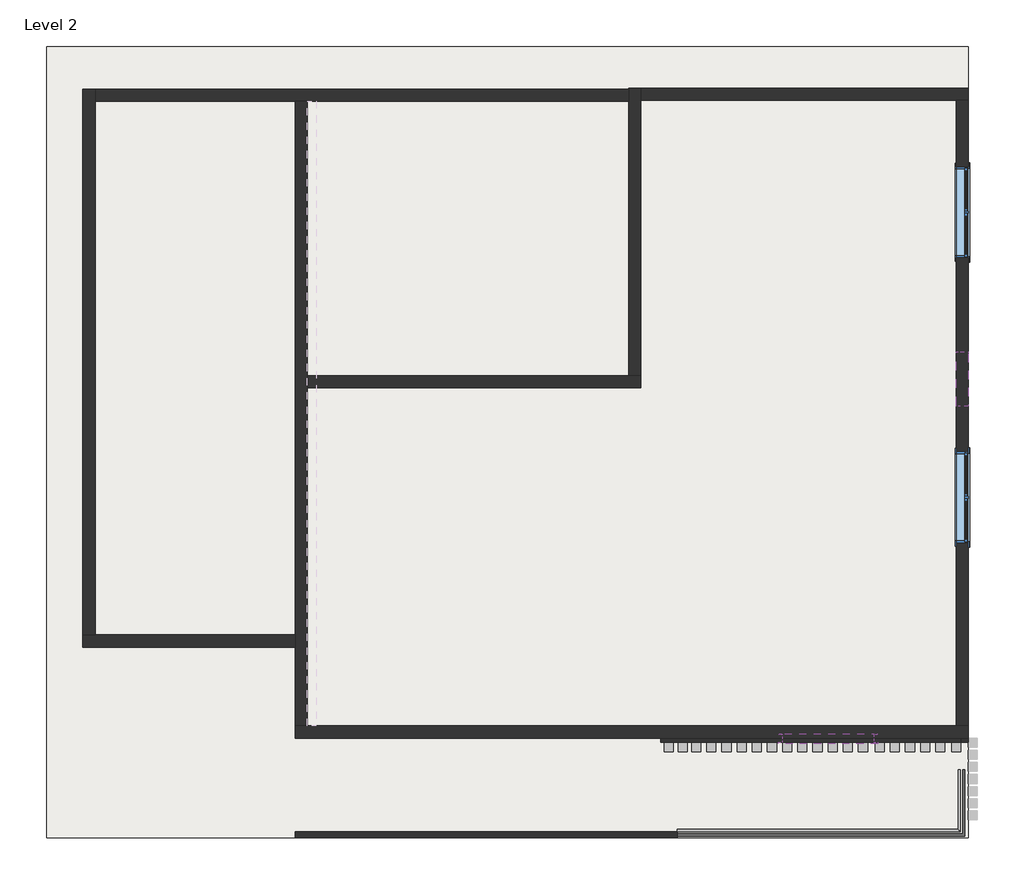
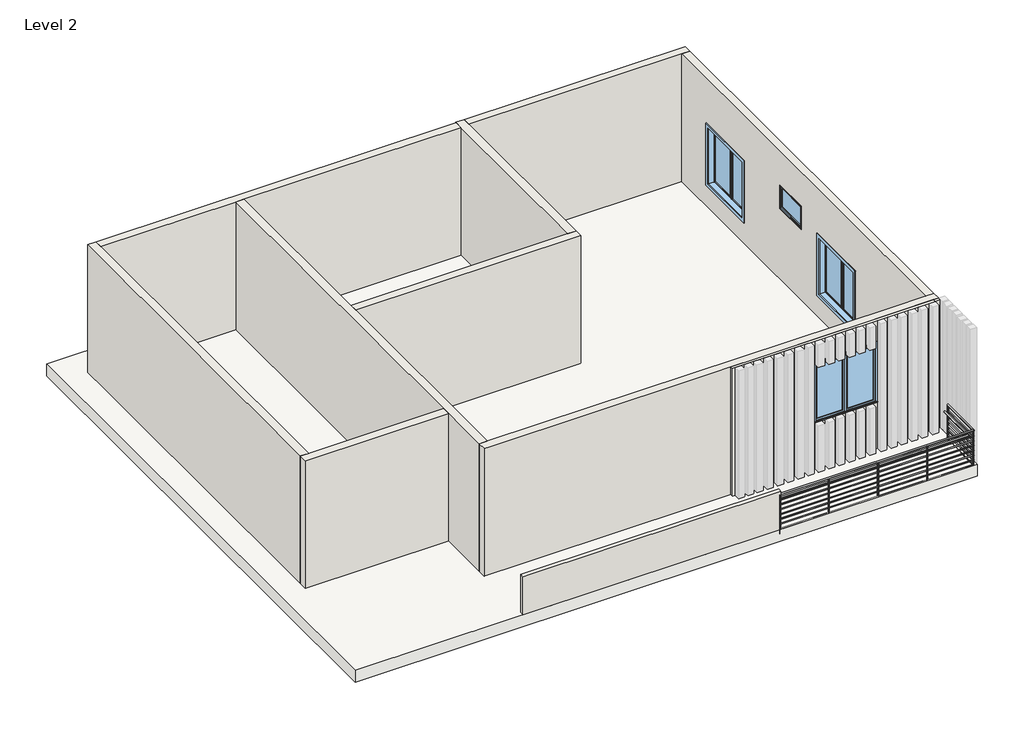
# One storey, part 1 of 2: 12 walls, 4 windows, 1 railing, 1 roof.
"""IFC4 building model written with IfcOpenShell, lengths in millimetres."""

from ifc_helpers import new_model, si_unit, point, frame, frame_2d, origin, place, context, project, spatial, polyline, circle_curve, ellipse_curve, trimmed, segment, composite_curve, outline, extrude, faceted_brep, transform, mapped, element, save
from ifc_brep_helpers import plane_surface, cylinder_surface, advanced_brep
from components import window_514a67b1, window_26183f51, window_57c3ee1c

model = new_model("IFC4")

# Units and contexts
model_context = context("Model", 3, world=origin())
ifc_project = project(units=[si_unit("LENGTHUNIT", "METRE", prefix="MILLI")], contexts=[model_context])

# Site, building, storey
site = spatial("IfcSite", under=ifc_project)
building = spatial("IfcBuilding", under=site)
storey = spatial("IfcBuildingStorey", under=building, Name="Level 2", Elevation=3657.6)

# Railing
placement = place(None, origin())
element("IfcRailing", 1, ObjectType="Guardrail - Pipe", at=placement, inside=storey, context=model_context, shape_type="SolidModel", body=[
    advanced_brep(
    [(1187.0250851, -2426.4018013, 4705.35), (1187.0250851, -2388.3018013, 4705.35), (5930.4750851, -2426.4018013, 4705.35), (5892.3750851, -2388.3018013, 4705.35), (5930.4750851, -1391.3518013, 4705.35), (5892.3750851, -1391.3518013, 4705.35)],
    [
        (0, 1, circle_curve(frame((1187.0250851, -2407.3518013, 4705.35), z_axis=(-1.0, 0.0, 0.0), x_axis=(0.0, 1.0, 0.0)), 19.05)),
        (1, 0, circle_curve(frame((1187.0250851, -2407.3518013, 4705.35), z_axis=(-1.0, 0.0, 0.0), x_axis=(0.0, 1.0, 0.0)), 19.05)),
        (0, 2),
        (2, 3, ellipse_curve(frame((5911.4250851, -2407.3518013, 4705.35), z_axis=(-0.7071067811865492, -0.7071067811865457, 0.0), x_axis=(-0.7071067811865458, 0.7071067811865491, 0.0)), 26.9407684, 19.05)),
        (3, 1),
        (3, 2, ellipse_curve(frame((5911.4250851, -2407.3518013, 4705.35), z_axis=(-0.7071067811865492, -0.7071067811865457, 0.0), x_axis=(-0.7071067811865458, 0.7071067811865491, 0.0)), 26.9407684, 19.05)),
        (4, 5, circle_curve(frame((5911.4250851, -1391.3518013, 4705.35), z_axis=(0.0, 1.0, 0.0), x_axis=(-1.0, 0.0, 0.0)), 19.05)),
        (5, 4, circle_curve(frame((5911.4250851, -1391.3518013, 4705.35), z_axis=(0.0, 1.0, 0.0), x_axis=(-1.0, 0.0, 0.0)), 19.05)),
        (2, 4),
        (5, 3),
    ],
    [
        plane_surface(frame((1187.0250851, -2407.3518013, 4724.4), z_axis=(-1.0, 0.0, 0.0), x_axis=(0.0, 1.0, 0.0))),
        cylinder_surface(frame((1187.0250851, -2407.3518013, 4705.35), z_axis=(-1.0, 0.0, 0.0), x_axis=(0.0, 1.0, 0.0)), 19.05),
        plane_surface(frame((5911.4250851, -1391.3518013, 4724.4), z_axis=(0.0, 1.0, 0.0), x_axis=(0.0, 0.0, 1.0))),
        cylinder_surface(frame((5911.4250851, -2407.3518013, 4705.35), z_axis=(0.0, -1.0, 0.0), x_axis=(-1.0, 0.0, 0.0)), 19.05),
    ],
    [
        (0, [[1, 2]]),
        (1, [[-1, 3, 4, 5]]),
        (1, [[-2, -5, 6, -3]]),
        (2, [[7, 8]]),
        (3, [[-4, 9, -8, 10]]),
        (3, [[-6, -10, -7, -9]]),
    ],
),
    advanced_brep(
    [(1187.0250851, -2502.6018013, 4857.75), (1187.0250851, -2464.5018013, 4857.75), (6006.6750851, -1391.3518013, 4857.75), (5968.5750851, -1391.3518013, 4857.75), (6006.6750851, -2502.6018013, 4857.75), (5968.5750851, -2464.5018013, 4857.75)],
    [
        (0, 1, circle_curve(frame((1187.0250851, -2483.5518013, 4857.75), z_axis=(-1.0, 0.0, 0.0), x_axis=(0.0, 1.0, 0.0)), 19.05)),
        (1, 0, circle_curve(frame((1187.0250851, -2483.5518013, 4857.75), z_axis=(-1.0, 0.0, 0.0), x_axis=(0.0, 1.0, 0.0)), 19.05)),
        (2, 3, circle_curve(frame((5987.6250851, -1391.3518013, 4857.75), z_axis=(0.0, 1.0, 0.0), x_axis=(-1.0, 0.0, 0.0)), 19.05)),
        (3, 2, circle_curve(frame((5987.6250851, -1391.3518013, 4857.75), z_axis=(0.0, 1.0, 0.0), x_axis=(-1.0, 0.0, 0.0)), 19.05)),
        (0, 4),
        (4, 5, ellipse_curve(frame((5987.6250851, -2483.5518013, 4857.75), z_axis=(-0.7071067811865492, -0.7071067811865457, 0.0), x_axis=(-0.7071067811865458, 0.7071067811865491, 0.0)), 26.9407684, 19.05)),
        (5, 1),
        (5, 4, ellipse_curve(frame((5987.6250851, -2483.5518013, 4857.75), z_axis=(-0.7071067811865492, -0.7071067811865457, 0.0), x_axis=(-0.7071067811865458, 0.7071067811865491, 0.0)), 26.9407684, 19.05)),
        (4, 2),
        (3, 5),
    ],
    [
        plane_surface(frame((1187.0250851, -2483.5518013, 4876.8), z_axis=(-1.0, 0.0, 0.0), x_axis=(0.0, 1.0, 0.0))),
        plane_surface(frame((5987.6250851, -1391.3518013, 4876.8), z_axis=(0.0, 1.0, 0.0), x_axis=(0.0, 0.0, 1.0))),
        cylinder_surface(frame((1187.0250851, -2483.5518013, 4857.75), z_axis=(-1.0, 0.0, 0.0), x_axis=(0.0, 1.0, 0.0)), 19.05),
        cylinder_surface(frame((5987.6250851, -2483.5518013, 4857.75), z_axis=(0.0, -1.0, 0.0), x_axis=(-1.0, 0.0, 0.0)), 19.05),
    ],
    [
        (0, [[1, 2]]),
        (1, [[3, 4]]),
        (2, [[-1, 5, 6, 7]]),
        (2, [[-2, -7, 8, -5]]),
        (3, [[-6, 9, -4, 10]]),
        (3, [[-8, -10, -3, -9]]),
    ],
),
    advanced_brep(
    [(1187.0250851, -2470.8518013, 4711.7), (1187.0250851, -2496.2518013, 4711.7), (5974.9250851, -2470.8518013, 4711.7), (6000.3250851, -2496.2518013, 4711.7), (5974.9250851, -1391.3518013, 4711.7), (6000.3250851, -1391.3518013, 4711.7)],
    [
        (0, 1, circle_curve(frame((1187.0250851, -2483.5518013, 4711.7), z_axis=(-1.0, 0.0, 0.0), x_axis=(0.0, -1.0, 0.0)), 12.7)),
        (1, 0, circle_curve(frame((1187.0250851, -2483.5518013, 4711.7), z_axis=(-1.0, 0.0, 0.0), x_axis=(0.0, -1.0, 0.0)), 12.7)),
        (0, 2),
        (2, 3, ellipse_curve(frame((5987.6250851, -2483.5518013, 4711.7), z_axis=(-0.7071067811865492, -0.7071067811865457, 0.0), x_axis=(-0.7071067811865458, 0.7071067811865491, 0.0)), 17.9605122, 12.7)),
        (3, 1),
        (3, 2, ellipse_curve(frame((5987.6250851, -2483.5518013, 4711.7), z_axis=(-0.7071067811865492, -0.7071067811865457, 0.0), x_axis=(-0.7071067811865458, 0.7071067811865491, 0.0)), 17.9605122, 12.7)),
        (4, 5, circle_curve(frame((5987.6250851, -1391.3518013, 4711.7), z_axis=(0.0, 1.0, 0.0), x_axis=(1.0, 0.0, 0.0)), 12.7)),
        (5, 4, circle_curve(frame((5987.6250851, -1391.3518013, 4711.7), z_axis=(0.0, 1.0, 0.0), x_axis=(1.0, 0.0, 0.0)), 12.7)),
        (2, 4),
        (5, 3),
    ],
    [
        plane_surface(frame((1187.0250851, -2483.5518013, 4724.4), z_axis=(-1.0, 0.0, 0.0), x_axis=(0.0, 1.0, 0.0))),
        cylinder_surface(frame((1187.0250851, -2483.5518013, 4711.7), z_axis=(-1.0, 0.0, 0.0), x_axis=(0.0, -1.0, 0.0)), 12.7),
        plane_surface(frame((5987.6250851, -1391.3518013, 4724.4), z_axis=(0.0, 1.0, 0.0), x_axis=(0.0, 0.0, 1.0))),
        cylinder_surface(frame((5987.6250851, -2483.5518013, 4711.7), z_axis=(0.0, -1.0, 0.0), x_axis=(1.0, 0.0, 0.0)), 12.7),
    ],
    [
        (0, [[1, 2]]),
        (1, [[-1, 3, 4, 5]]),
        (1, [[-2, -5, 6, -3]]),
        (2, [[7, 8]]),
        (3, [[-4, 9, -8, 10]]),
        (3, [[-6, -10, -7, -9]]),
    ],
),
    advanced_brep(
    [(1187.0250851, -2470.8518013, 4584.7), (1187.0250851, -2496.2518013, 4584.7), (5974.9250851, -2470.8518013, 4584.7), (6000.3250851, -2496.2518013, 4584.7), (5974.9250851, -1391.3518013, 4584.7), (6000.3250851, -1391.3518013, 4584.7)],
    [
        (0, 1, circle_curve(frame((1187.0250851, -2483.5518013, 4584.7), z_axis=(-1.0, 0.0, 0.0), x_axis=(0.0, -1.0, 0.0)), 12.7)),
        (1, 0, circle_curve(frame((1187.0250851, -2483.5518013, 4584.7), z_axis=(-1.0, 0.0, 0.0), x_axis=(0.0, -1.0, 0.0)), 12.7)),
        (0, 2),
        (2, 3, ellipse_curve(frame((5987.6250851, -2483.5518013, 4584.7), z_axis=(-0.7071067811865492, -0.7071067811865457, 0.0), x_axis=(-0.7071067811865458, 0.7071067811865491, 0.0)), 17.9605122, 12.7)),
        (3, 1),
        (3, 2, ellipse_curve(frame((5987.6250851, -2483.5518013, 4584.7), z_axis=(-0.7071067811865492, -0.7071067811865457, 0.0), x_axis=(-0.7071067811865458, 0.7071067811865491, 0.0)), 17.9605122, 12.7)),
        (4, 5, circle_curve(frame((5987.6250851, -1391.3518013, 4584.7), z_axis=(0.0, 1.0, 0.0), x_axis=(1.0, 0.0, 0.0)), 12.7)),
        (5, 4, circle_curve(frame((5987.6250851, -1391.3518013, 4584.7), z_axis=(0.0, 1.0, 0.0), x_axis=(1.0, 0.0, 0.0)), 12.7)),
        (2, 4),
        (5, 3),
    ],
    [
        plane_surface(frame((1187.0250851, -2483.5518013, 4597.4), z_axis=(-1.0, 0.0, 0.0), x_axis=(0.0, 1.0, 0.0))),
        cylinder_surface(frame((1187.0250851, -2483.5518013, 4584.7), z_axis=(-1.0, 0.0, 0.0), x_axis=(0.0, -1.0, 0.0)), 12.7),
        plane_surface(frame((5987.6250851, -1391.3518013, 4597.4), z_axis=(0.0, 1.0, 0.0), x_axis=(0.0, 0.0, 1.0))),
        cylinder_surface(frame((5987.6250851, -2483.5518013, 4584.7), z_axis=(0.0, -1.0, 0.0), x_axis=(1.0, 0.0, 0.0)), 12.7),
    ],
    [
        (0, [[1, 2]]),
        (1, [[-1, 3, 4, 5]]),
        (1, [[-2, -5, 6, -3]]),
        (2, [[7, 8]]),
        (3, [[-4, 9, -8, 10]]),
        (3, [[-6, -10, -7, -9]]),
    ],
),
    advanced_brep(
    [(1187.0250851, -2470.8518013, 4457.7), (1187.0250851, -2496.2518013, 4457.7), (5974.9250851, -2470.8518013, 4457.7), (6000.3250851, -2496.2518013, 4457.7), (5974.9250851, -1391.3518013, 4457.7), (6000.3250851, -1391.3518013, 4457.7)],
    [
        (0, 1, circle_curve(frame((1187.0250851, -2483.5518013, 4457.7), z_axis=(-1.0, 0.0, 0.0), x_axis=(0.0, -1.0, 0.0)), 12.7)),
        (1, 0, circle_curve(frame((1187.0250851, -2483.5518013, 4457.7), z_axis=(-1.0, 0.0, 0.0), x_axis=(0.0, -1.0, 0.0)), 12.7)),
        (0, 2),
        (2, 3, ellipse_curve(frame((5987.6250851, -2483.5518013, 4457.7), z_axis=(-0.7071067811865492, -0.7071067811865457, 0.0), x_axis=(-0.7071067811865458, 0.7071067811865491, 0.0)), 17.9605122, 12.7)),
        (3, 1),
        (3, 2, ellipse_curve(frame((5987.6250851, -2483.5518013, 4457.7), z_axis=(-0.7071067811865492, -0.7071067811865457, 0.0), x_axis=(-0.7071067811865458, 0.7071067811865491, 0.0)), 17.9605122, 12.7)),
        (4, 5, circle_curve(frame((5987.6250851, -1391.3518013, 4457.7), z_axis=(0.0, 1.0, 0.0), x_axis=(1.0, 0.0, 0.0)), 12.7)),
        (5, 4, circle_curve(frame((5987.6250851, -1391.3518013, 4457.7), z_axis=(0.0, 1.0, 0.0), x_axis=(1.0, 0.0, 0.0)), 12.7)),
        (2, 4),
        (5, 3),
    ],
    [
        plane_surface(frame((1187.0250851, -2483.5518013, 4470.4), z_axis=(-1.0, 0.0, 0.0), x_axis=(0.0, 1.0, 0.0))),
        cylinder_surface(frame((1187.0250851, -2483.5518013, 4457.7), z_axis=(-1.0, 0.0, 0.0), x_axis=(0.0, -1.0, 0.0)), 12.7),
        plane_surface(frame((5987.6250851, -1391.3518013, 4470.4), z_axis=(0.0, 1.0, 0.0), x_axis=(0.0, 0.0, 1.0))),
        cylinder_surface(frame((5987.6250851, -2483.5518013, 4457.7), z_axis=(0.0, -1.0, 0.0), x_axis=(1.0, 0.0, 0.0)), 12.7),
    ],
    [
        (0, [[1, 2]]),
        (1, [[-1, 3, 4, 5]]),
        (1, [[-2, -5, 6, -3]]),
        (2, [[7, 8]]),
        (3, [[-4, 9, -8, 10]]),
        (3, [[-6, -10, -7, -9]]),
    ],
),
    advanced_brep(
    [(1187.0250851, -2470.8518013, 4330.7), (1187.0250851, -2496.2518013, 4330.7), (5974.9250851, -2470.8518013, 4330.7), (6000.3250851, -2496.2518013, 4330.7), (5974.9250851, -1391.3518013, 4330.7), (6000.3250851, -1391.3518013, 4330.7)],
    [
        (0, 1, circle_curve(frame((1187.0250851, -2483.5518013, 4330.7), z_axis=(-1.0, 0.0, 0.0), x_axis=(0.0, -1.0, 0.0)), 12.7)),
        (1, 0, circle_curve(frame((1187.0250851, -2483.5518013, 4330.7), z_axis=(-1.0, 0.0, 0.0), x_axis=(0.0, -1.0, 0.0)), 12.7)),
        (0, 2),
        (2, 3, ellipse_curve(frame((5987.6250851, -2483.5518013, 4330.7), z_axis=(-0.7071067811865492, -0.7071067811865457, 0.0), x_axis=(-0.7071067811865458, 0.7071067811865491, 0.0)), 17.9605122, 12.7)),
        (3, 1),
        (3, 2, ellipse_curve(frame((5987.6250851, -2483.5518013, 4330.7), z_axis=(-0.7071067811865492, -0.7071067811865457, 0.0), x_axis=(-0.7071067811865458, 0.7071067811865491, 0.0)), 17.9605122, 12.7)),
        (4, 5, circle_curve(frame((5987.6250851, -1391.3518013, 4330.7), z_axis=(0.0, 1.0, 0.0), x_axis=(1.0, 0.0, 0.0)), 12.7)),
        (5, 4, circle_curve(frame((5987.6250851, -1391.3518013, 4330.7), z_axis=(0.0, 1.0, 0.0), x_axis=(1.0, 0.0, 0.0)), 12.7)),
        (2, 4),
        (5, 3),
    ],
    [
        plane_surface(frame((1187.0250851, -2483.5518013, 4343.4), z_axis=(-1.0, 0.0, 0.0), x_axis=(0.0, 1.0, 0.0))),
        cylinder_surface(frame((1187.0250851, -2483.5518013, 4330.7), z_axis=(-1.0, 0.0, 0.0), x_axis=(0.0, -1.0, 0.0)), 12.7),
        plane_surface(frame((5987.6250851, -1391.3518013, 4343.4), z_axis=(0.0, 1.0, 0.0), x_axis=(0.0, 0.0, 1.0))),
        cylinder_surface(frame((5987.6250851, -2483.5518013, 4330.7), z_axis=(0.0, -1.0, 0.0), x_axis=(1.0, 0.0, 0.0)), 12.7),
    ],
    [
        (0, [[1, 2]]),
        (1, [[-1, 3, 4, 5]]),
        (1, [[-2, -5, 6, -3]]),
        (2, [[7, 8]]),
        (3, [[-4, 9, -8, 10]]),
        (3, [[-6, -10, -7, -9]]),
    ],
),
    advanced_brep(
    [(1187.0250851, -2470.8518013, 4203.7), (1187.0250851, -2496.2518013, 4203.7), (5974.9250851, -2470.8518013, 4203.7), (6000.3250851, -2496.2518013, 4203.7), (5974.9250851, -1391.3518013, 4203.7), (6000.3250851, -1391.3518013, 4203.7)],
    [
        (0, 1, circle_curve(frame((1187.0250851, -2483.5518013, 4203.7), z_axis=(-1.0, 0.0, 0.0), x_axis=(0.0, -1.0, 0.0)), 12.7)),
        (1, 0, circle_curve(frame((1187.0250851, -2483.5518013, 4203.7), z_axis=(-1.0, 0.0, 0.0), x_axis=(0.0, -1.0, 0.0)), 12.7)),
        (0, 2),
        (2, 3, ellipse_curve(frame((5987.6250851, -2483.5518013, 4203.7), z_axis=(-0.7071067811865492, -0.7071067811865457, 0.0), x_axis=(-0.7071067811865458, 0.7071067811865491, 0.0)), 17.9605122, 12.7)),
        (3, 1),
        (3, 2, ellipse_curve(frame((5987.6250851, -2483.5518013, 4203.7), z_axis=(-0.7071067811865492, -0.7071067811865457, 0.0), x_axis=(-0.7071067811865458, 0.7071067811865491, 0.0)), 17.9605122, 12.7)),
        (4, 5, circle_curve(frame((5987.6250851, -1391.3518013, 4203.7), z_axis=(0.0, 1.0, 0.0), x_axis=(1.0, 0.0, 0.0)), 12.7)),
        (5, 4, circle_curve(frame((5987.6250851, -1391.3518013, 4203.7), z_axis=(0.0, 1.0, 0.0), x_axis=(1.0, 0.0, 0.0)), 12.7)),
        (2, 4),
        (5, 3),
    ],
    [
        plane_surface(frame((1187.0250851, -2483.5518013, 4216.4), z_axis=(-1.0, 0.0, 0.0), x_axis=(0.0, 1.0, 0.0))),
        cylinder_surface(frame((1187.0250851, -2483.5518013, 4203.7), z_axis=(-1.0, 0.0, 0.0), x_axis=(0.0, -1.0, 0.0)), 12.7),
        plane_surface(frame((5987.6250851, -1391.3518013, 4216.4), z_axis=(0.0, 1.0, 0.0), x_axis=(0.0, 0.0, 1.0))),
        cylinder_surface(frame((5987.6250851, -2483.5518013, 4203.7), z_axis=(0.0, -1.0, 0.0), x_axis=(1.0, 0.0, 0.0)), 12.7),
    ],
    [
        (0, [[1, 2]]),
        (1, [[-1, 3, 4, 5]]),
        (1, [[-2, -5, 6, -3]]),
        (2, [[7, 8]]),
        (3, [[-4, 9, -8, 10]]),
        (3, [[-6, -10, -7, -9]]),
    ],
),
    advanced_brep(
    [(1187.0250851, -2470.8518013, 4076.7), (1187.0250851, -2496.2518013, 4076.7), (5974.9250851, -2470.8518013, 4076.7), (6000.3250851, -2496.2518013, 4076.7), (5974.9250851, -1391.3518013, 4076.7), (6000.3250851, -1391.3518013, 4076.7)],
    [
        (0, 1, circle_curve(frame((1187.0250851, -2483.5518013, 4076.7), z_axis=(-1.0, 0.0, 0.0), x_axis=(0.0, -1.0, 0.0)), 12.7)),
        (1, 0, circle_curve(frame((1187.0250851, -2483.5518013, 4076.7), z_axis=(-1.0, 0.0, 0.0), x_axis=(0.0, -1.0, 0.0)), 12.7)),
        (0, 2),
        (2, 3, ellipse_curve(frame((5987.6250851, -2483.5518013, 4076.7), z_axis=(-0.7071067811865492, -0.7071067811865457, 0.0), x_axis=(-0.7071067811865458, 0.7071067811865491, 0.0)), 17.9605122, 12.7)),
        (3, 1),
        (3, 2, ellipse_curve(frame((5987.6250851, -2483.5518013, 4076.7), z_axis=(-0.7071067811865492, -0.7071067811865457, 0.0), x_axis=(-0.7071067811865458, 0.7071067811865491, 0.0)), 17.9605122, 12.7)),
        (4, 5, circle_curve(frame((5987.6250851, -1391.3518013, 4076.7), z_axis=(0.0, 1.0, 0.0), x_axis=(1.0, 0.0, 0.0)), 12.7)),
        (5, 4, circle_curve(frame((5987.6250851, -1391.3518013, 4076.7), z_axis=(0.0, 1.0, 0.0), x_axis=(1.0, 0.0, 0.0)), 12.7)),
        (2, 4),
        (5, 3),
    ],
    [
        plane_surface(frame((1187.0250851, -2483.5518013, 4089.4), z_axis=(-1.0, 0.0, 0.0), x_axis=(0.0, 1.0, 0.0))),
        cylinder_surface(frame((1187.0250851, -2483.5518013, 4076.7), z_axis=(-1.0, 0.0, 0.0), x_axis=(0.0, -1.0, 0.0)), 12.7),
        plane_surface(frame((5987.6250851, -1391.3518013, 4089.4), z_axis=(0.0, 1.0, 0.0), x_axis=(0.0, 0.0, 1.0))),
        cylinder_surface(frame((5987.6250851, -2483.5518013, 4076.7), z_axis=(0.0, -1.0, 0.0), x_axis=(1.0, 0.0, 0.0)), 12.7),
    ],
    [
        (0, [[1, 2]]),
        (1, [[-1, 3, 4, 5]]),
        (1, [[-2, -5, 6, -3]]),
        (2, [[7, 8]]),
        (3, [[-4, 9, -8, 10]]),
        (3, [[-6, -10, -7, -9]]),
    ],
),
    advanced_brep(
    [(1187.0250851, -2470.8518013, 3949.7), (1187.0250851, -2496.2518013, 3949.7), (5974.9250851, -2470.8518013, 3949.7), (6000.3250851, -2496.2518013, 3949.7), (5974.9250851, -1391.3518013, 3949.7), (6000.3250851, -1391.3518013, 3949.7)],
    [
        (0, 1, circle_curve(frame((1187.0250851, -2483.5518013, 3949.7), z_axis=(-1.0, 0.0, 0.0), x_axis=(0.0, -1.0, 0.0)), 12.7)),
        (1, 0, circle_curve(frame((1187.0250851, -2483.5518013, 3949.7), z_axis=(-1.0, 0.0, 0.0), x_axis=(0.0, -1.0, 0.0)), 12.7)),
        (0, 2),
        (2, 3, ellipse_curve(frame((5987.6250851, -2483.5518013, 3949.7), z_axis=(-0.7071067811865492, -0.7071067811865457, 0.0), x_axis=(-0.7071067811865458, 0.7071067811865491, 0.0)), 17.9605122, 12.7)),
        (3, 1),
        (3, 2, ellipse_curve(frame((5987.6250851, -2483.5518013, 3949.7), z_axis=(-0.7071067811865492, -0.7071067811865457, 0.0), x_axis=(-0.7071067811865458, 0.7071067811865491, 0.0)), 17.9605122, 12.7)),
        (4, 5, circle_curve(frame((5987.6250851, -1391.3518013, 3949.7), z_axis=(0.0, 1.0, 0.0), x_axis=(1.0, 0.0, 0.0)), 12.7)),
        (5, 4, circle_curve(frame((5987.6250851, -1391.3518013, 3949.7), z_axis=(0.0, 1.0, 0.0), x_axis=(1.0, 0.0, 0.0)), 12.7)),
        (2, 4),
        (5, 3),
    ],
    [
        plane_surface(frame((1187.0250851, -2483.5518013, 3962.4), z_axis=(-1.0, 0.0, 0.0), x_axis=(0.0, 1.0, 0.0))),
        cylinder_surface(frame((1187.0250851, -2483.5518013, 3949.7), z_axis=(-1.0, 0.0, 0.0), x_axis=(0.0, -1.0, 0.0)), 12.7),
        plane_surface(frame((5987.6250851, -1391.3518013, 3962.4), z_axis=(0.0, 1.0, 0.0), x_axis=(0.0, 0.0, 1.0))),
        cylinder_surface(frame((5987.6250851, -2483.5518013, 3949.7), z_axis=(0.0, -1.0, 0.0), x_axis=(1.0, 0.0, 0.0)), 12.7),
    ],
    [
        (0, [[1, 2]]),
        (1, [[-1, 3, 4, 5]]),
        (1, [[-2, -5, 6, -3]]),
        (2, [[7, 8]]),
        (3, [[-4, 9, -8, 10]]),
        (3, [[-6, -10, -7, -9]]),
    ],
),
    extrude(outline(composite_curve([segment(trimmed(circle_curve(frame_2d((4844.6250851, -2483.5518013)), 12.7), [point((4844.6250851, -2470.8518013))], [point((4844.6250851, -2496.2518013))], False, "CARTESIAN"), True, "CONTINUOUS"), segment(trimmed(circle_curve(frame_2d((4844.6250851, -2483.5518013)), 12.7), [point((4844.6250851, -2496.2518013))], [point((4844.6250851, -2470.8518013))], False, "CARTESIAN"), True, "CONTINUOUS")], self_intersect=False)), frame((0.0, 0.0, 3810.0), z_axis=(0.0, 0.0, 1.0), x_axis=(1.0, 0.0, 0.0)), (0.0, 0.0, 1.0), 1028.7),
    extrude(outline(composite_curve([segment(trimmed(circle_curve(frame_2d((3625.4250851, -2483.5518013)), 12.7), [point((3625.4250851, -2470.8518013))], [point((3625.4250851, -2496.2518013))], False, "CARTESIAN"), True, "CONTINUOUS"), segment(trimmed(circle_curve(frame_2d((3625.4250851, -2483.5518013)), 12.7), [point((3625.4250851, -2496.2518013))], [point((3625.4250851, -2470.8518013))], False, "CARTESIAN"), True, "CONTINUOUS")], self_intersect=False)), frame((0.0, 0.0, 3810.0), z_axis=(0.0, 0.0, 1.0), x_axis=(1.0, 0.0, 0.0)), (0.0, 0.0, 1.0), 1028.7),
    extrude(outline(composite_curve([segment(trimmed(circle_curve(frame_2d((2406.2250851, -2483.5518013)), 12.7), [point((2406.2250851, -2470.8518013))], [point((2406.2250851, -2496.2518013))], False, "CARTESIAN"), True, "CONTINUOUS"), segment(trimmed(circle_curve(frame_2d((2406.2250851, -2483.5518013)), 12.7), [point((2406.2250851, -2496.2518013))], [point((2406.2250851, -2470.8518013))], False, "CARTESIAN"), True, "CONTINUOUS")], self_intersect=False)), frame((0.0, 0.0, 3810.0), z_axis=(0.0, 0.0, 1.0), x_axis=(1.0, 0.0, 0.0)), (0.0, 0.0, 1.0), 1028.7),
    extrude(outline(composite_curve([segment(trimmed(circle_curve(frame_2d((5987.6250851, -2483.5518013)), 12.7), [point((5987.6250851, -2470.8518013))], [point((5987.6250851, -2496.2518013))], False, "CARTESIAN"), True, "CONTINUOUS"), segment(trimmed(circle_curve(frame_2d((5987.6250851, -2483.5518013)), 12.7), [point((5987.6250851, -2496.2518013))], [point((5987.6250851, -2470.8518013))], False, "CARTESIAN"), True, "CONTINUOUS")], self_intersect=False)), frame((0.0, 0.0, 3810.0), z_axis=(0.0, 0.0, 1.0), x_axis=(1.0, 0.0, 0.0)), (0.0, 0.0, 1.0), 1028.7),
    extrude(outline(composite_curve([segment(trimmed(circle_curve(frame_2d((5987.6250851, -1404.0518013)), 12.7), [point((5974.9250851, -1404.0518013))], [point((6000.3250851, -1404.0518013))], False, "CARTESIAN"), True, "CONTINUOUS"), segment(trimmed(circle_curve(frame_2d((5987.6250851, -1404.0518013)), 12.7), [point((6000.3250851, -1404.0518013))], [point((5974.9250851, -1404.0518013))], False, "CARTESIAN"), True, "CONTINUOUS")], self_intersect=False)), frame((0.0, 0.0, 3810.0), z_axis=(0.0, 0.0, 1.0), x_axis=(1.0, 0.0, 0.0)), (0.0, 0.0, 1.0), 1028.7),
    extrude(outline(composite_curve([segment(trimmed(circle_curve(frame_2d((1199.7250851, -2483.5518013)), 12.7), [point((1199.7250851, -2470.8518013))], [point((1199.7250851, -2496.2518013))], False, "CARTESIAN"), True, "CONTINUOUS"), segment(trimmed(circle_curve(frame_2d((1199.7250851, -2483.5518013)), 12.7), [point((1199.7250851, -2496.2518013))], [point((1199.7250851, -2470.8518013))], False, "CARTESIAN"), True, "CONTINUOUS")], self_intersect=False)), frame((0.0, 0.0, 3810.0), z_axis=(0.0, 0.0, 1.0), x_axis=(1.0, 0.0, 0.0)), (0.0, 0.0, 1.0), 1028.7),
])

# Roof
element("IfcRoof", 2, ObjectType="Generic - 12\"", at=placement, inside=storey, context=model_context, shape_type="SweptSolid", body=[
    extrude(outline(polyline([(-9379.3749149, 10724.4481987), (6063.8250851, 10724.4481987), (6063.8250851, -2534.3518013), (-9379.3749149, -2534.3518013), (-9379.3749149, 10724.4481987)])), frame((0.0, 0.0, 3657.6), z_axis=(0.0, 0.0, 1.0), x_axis=(1.0, 0.0, 0.0)), (0.0, 0.0, 1.0), 304.8),
])

# Walls
element("IfcWall", 3, ObjectType="Generic - 4\" Brick", at=placement, inside=storey, context=model_context, shape_type="SweptSolid", body=[
    extrude(outline(polyline([(1187.0250851, -2534.3518013), (-5213.7749149, -2534.3518013), (-5213.7749149, -2432.7518013), (1187.0250851, -2432.7518013), (1187.0250851, -2534.3518013)])), frame((0.0, 0.0, 3962.4), z_axis=(0.0, 0.0, 1.0), x_axis=(1.0, 0.0, 0.0)), (0.0, 0.0, 1.0), 1000.26952),
])
element("IfcWall", 4, ObjectType="Generic - 5\"", at=placement, inside=storey, context=model_context, shape_type="SweptSolid", body=[
    extrude(outline(polyline([(5936.8250851, -934.1518013), (5936.8250851, -860.9451257), (6063.8250851, -860.9451257), (6063.8250851, -934.1518013), (5936.8250851, -934.1518013)])), frame((0.0, 0.0, 3657.6), z_axis=(0.0, 0.0, 1.0), x_axis=(1.0, 0.0, 0.0)), (0.0, 0.0, 1.0), 3657.6),
])
element("IfcWall", 5, ObjectType="Generic - 5\"", at=placement, inside=storey, context=model_context, shape_type="Brep", body=[
    faceted_brep([(5936.8250851, -807.1518013, 3657.6), (907.6250851, -807.1518013, 3657.6), (907.6250851, -807.1518013, 7315.2), (5936.8250851, -807.1518013, 7315.2), (2952.3250851, -807.1518013, 6714.2723515), (2952.3250851, -807.1518013, 5190.2723515), (4476.3250851, -807.1518013, 5190.2723515), (4476.3250851, -807.1518013, 6714.2723515), (5936.8250851, -934.1518013, 3657.6), (5936.8250851, -934.1518013, 7315.2), (907.6250851, -934.1518013, 7315.2), (907.6250851, -934.1518013, 3657.6), (2952.3250851, -934.1518013, 6714.2723515), (4476.3250851, -934.1518013, 6714.2723515), (4476.3250851, -934.1518013, 5190.2723515), (2952.3250851, -934.1518013, 5190.2723515), (5936.8250851, -860.9451257, 7315.2), (5936.8250851, -860.9451257, 3657.6)], [[[0, 1, 2, 3], [4, 5, 6, 7]], [[8, 9, 10, 11], [12, 13, 14, 15]], [[0, 3, 16, 9, 8, 17]], [[1, 0, 17, 8, 11]], [[2, 1, 11, 10]], [[3, 2, 10, 9, 16]], [[5, 4, 12, 15]], [[6, 5, 15, 14]], [[7, 6, 14, 13]], [[4, 7, 13, 12]]]),
])
element("IfcWall", 6, ObjectType="Generic - 8\"", at=placement, inside=storey, context=model_context, shape_type="Brep", body=[
    faceted_brep([(6063.8250851, -657.7451257, 3657.6), (5860.6250851, -657.7451257, 3657.6), (-5010.5749149, -657.7451257, 3657.6), (-5213.7749149, -657.7451257, 3657.6), (-5213.7749149, -657.7451257, 7315.2), (-5010.5749149, -657.7451257, 7315.2), (5016.0750851, -657.7451257, 7315.2), (5860.6250851, -657.7451257, 7315.2), (6063.8250851, -657.7451257, 7315.2), (6063.8250851, -860.9451257, 3657.6), (6063.8250851, -860.9451257, 7315.2), (5936.8250851, -860.9451257, 7315.2), (5016.0750851, -860.9451257, 7315.2), (-5086.7749149, -860.9451257, 7315.2), (-5213.7749149, -860.9451257, 7315.2), (-5213.7749149, -860.9451257, 3979.4508154), (-5213.7749149, -860.9451257, 3657.6), (5936.8250851, -860.9451257, 3657.6)], [[[0, 1, 2, 3, 4, 5, 6, 7, 8]], [[9, 10, 11, 12, 13, 14, 15, 16, 17]], [[3, 2, 1, 0, 9, 17, 16]], [[0, 8, 10, 9]], [[8, 7, 6, 5, 4, 14, 13, 12, 11, 10]], [[3, 16, 15, 14, 4]]]),
])
element("IfcWall", 7, ObjectType="Generic - 8\"", at=placement, inside=storey, context=model_context, shape_type="Brep", body=[
    faceted_brep([(-5010.5749149, -657.7451257, 7315.2), (-5010.5749149, -657.7451257, 3657.6), (-5010.5749149, 5006.4548743, 3657.6), (-5010.5749149, 5209.6548743, 3657.6), (-5010.5749149, 9807.0548743, 3657.6), (-5010.5749149, 9807.0548743, 7315.2), (-5010.5749149, 5209.6548743, 7315.2), (-5010.5749149, 5006.4548743, 7315.2), (-5213.7749149, -657.7451257, 3657.6), (-5213.7749149, -657.7451257, 7315.2), (-5213.7749149, 2.6548743, 7315.2), (-5213.7749149, 663.0548743, 7315.2), (-5213.7749149, 866.2548743, 7315.2), (-5213.7749149, 9807.0548743, 7315.2), (-5213.7749149, 9807.0548743, 3657.6), (-5213.7749149, 866.2548743, 3657.6), (-5213.7749149, 663.0548743, 3657.6)], [[[0, 1, 2, 3, 4, 5, 6, 7]], [[8, 9, 10, 11, 12, 13, 14, 15, 16]], [[4, 3, 2, 1, 8, 16, 15, 14]], [[5, 4, 14, 13]], [[0, 7, 6, 5, 13, 12, 11, 10, 9]], [[0, 9, 8, 1]]]),
])
element("IfcWall", 8, ObjectType="Generic - 8\"", at=placement, inside=storey, context=model_context, shape_type="Brep", body=[
    faceted_brep([(-8769.7749149, 663.0548743, 3657.6), (-5213.7749149, 663.0548743, 3657.6), (-5213.7749149, 663.0548743, 7315.2), (-8769.7749149, 663.0548743, 7315.2), (-8769.7749149, 866.2548743, 3657.6), (-8769.7749149, 866.2548743, 7315.2), (-8566.5749149, 866.2548743, 7315.2), (-5213.7749149, 866.2548743, 7315.2), (-5213.7749149, 866.2548743, 3657.6), (-8566.5749149, 866.2548743, 3657.6)], [[[0, 1, 2, 3]], [[4, 5, 6, 7, 8, 9]], [[1, 0, 4, 9, 8]], [[2, 1, 8, 7]], [[0, 3, 5, 4]], [[3, 2, 7, 6, 5]]]),
])
element("IfcWall", 9, ObjectType="Generic - 8\"", at=placement, inside=storey, context=model_context, shape_type="Brep", body=[
    faceted_brep([(-5010.5749149, 5006.4548743, 3657.6), (577.4250851, 5006.4548743, 3657.6), (577.4250851, 5006.4548743, 7315.2), (-5010.5749149, 5006.4548743, 7315.2), (-5010.5749149, 5209.6548743, 3657.6), (-5010.5749149, 5209.6548743, 7315.2), (374.2250851, 5209.6548743, 7315.2), (577.4250851, 5209.6548743, 7315.2), (577.4250851, 5209.6548743, 3657.6), (374.2250851, 5209.6548743, 3657.6)], [[[0, 1, 2, 3]], [[4, 5, 6, 7, 8, 9]], [[1, 0, 4, 9, 8]], [[0, 3, 5, 4]], [[2, 1, 8, 7]], [[3, 2, 7, 6, 5]]]),
])
element("IfcWall", 10, ObjectType="Generic - 8\"", at=placement, inside=storey, context=model_context, shape_type="Brep", body=[
    faceted_brep([(577.4250851, 5209.6548743, 3657.6), (577.4250851, 9826.1048743, 3657.6), (577.4250851, 10029.3048743, 3657.6), (577.4250851, 10029.3048743, 7315.2), (577.4250851, 9826.1048743, 7315.2), (577.4250851, 5209.6548743, 7315.2), (374.2250851, 5209.6548743, 3657.6), (374.2250851, 5209.6548743, 7315.2), (374.2250851, 9807.0548743, 7315.2), (374.2250851, 10010.2548743, 7315.2), (374.2250851, 10029.3048743, 7315.2), (374.2250851, 10029.3048743, 3657.6), (374.2250851, 10010.2548743, 3657.6), (374.2250851, 9807.0548743, 3657.6)], [[[0, 1, 2, 3, 4, 5]], [[6, 7, 8, 9, 10, 11, 12, 13]], [[2, 1, 0, 6, 13, 12, 11]], [[0, 5, 7, 6]], [[3, 2, 11, 10]], [[5, 4, 3, 10, 9, 8, 7]]]),
])
element("IfcWall", 11, ObjectType="Generic - 8\"", at=placement, inside=storey, context=model_context, shape_type="Brep", body=[
    faceted_brep([(577.4250851, 9826.1048743, 3657.6), (5860.6250851, 9826.1048743, 3657.6), (6063.8250851, 9826.1048743, 3657.6), (6063.8250851, 9826.1048743, 7315.2), (5860.6250851, 9826.1048743, 7315.2), (577.4250851, 9826.1048743, 7315.2), (577.4250851, 10029.3048743, 3657.6), (577.4250851, 10029.3048743, 7315.2), (6063.8250851, 10029.3048743, 7315.2), (6063.8250851, 10029.3048743, 3657.6)], [[[0, 1, 2, 3, 4, 5]], [[6, 7, 8, 9]], [[2, 1, 0, 6, 9]], [[0, 5, 7, 6]], [[3, 2, 9, 8]], [[5, 4, 3, 8, 7]]]),
])
element("IfcWall", 12, ObjectType="Generic - 8\"", at=placement, inside=storey, context=model_context, shape_type="SweptSolid", body=[
    extrude(outline(polyline([(9826.1048743, 3657.6), (-657.7451257, 3657.6), (-657.7451257, 7315.2), (9826.1048743, 7315.2), (9826.1048743, 3657.6)]), holes=[polyline([(5609.7048743, 6427.3756746), (4695.3048743, 6427.3756746), (4695.3048743, 5817.7756746), (5609.7048743, 5817.7756746), (5609.7048743, 6427.3756746)]), polyline([(2409.3048743, 6096.0), (2409.3048743, 4572.0), (3933.3048743, 4572.0), (3933.3048743, 6096.0), (2409.3048743, 6096.0)]), polyline([(7184.5048743, 6096.0), (7184.5048743, 4572.0), (8708.5048743, 4572.0), (8708.5048743, 6096.0), (7184.5048743, 6096.0)])]), frame((5860.6250851, 0.0, 0.0), z_axis=(1.0, 0.0, 0.0), x_axis=(0.0, 1.0, 0.0)), (0.0, 0.0, 1.0), 203.2),
])
element("IfcWall", 13, ObjectType="Generic - 8\"", at=placement, inside=storey, context=model_context, shape_type="Brep", body=[
    faceted_brep([(-8566.5749149, 866.2548743, 3657.6), (-8566.5749149, 9807.0548743, 3657.6), (-8566.5749149, 10010.2548743, 3657.6), (-8566.5749149, 10010.2548743, 7315.2), (-8566.5749149, 9807.0548743, 7315.2), (-8566.5749149, 866.2548743, 7315.2), (-8769.7749149, 866.2548743, 3657.6), (-8769.7749149, 866.2548743, 7315.2), (-8769.7749149, 10010.2548743, 7315.2), (-8769.7749149, 10010.2548743, 3657.6)], [[[0, 1, 2, 3, 4, 5]], [[6, 7, 8, 9]], [[2, 1, 0, 6, 9]], [[0, 5, 7, 6]], [[3, 2, 9, 8]], [[5, 4, 3, 8, 7]]]),
])
element("IfcWall", 14, ObjectType="Generic - 8\"", at=placement, inside=storey, context=model_context, shape_type="Brep", body=[
    faceted_brep([(-8566.5749149, 9807.0548743, 3657.6), (-5213.7749149, 9807.0548743, 3657.6), (-5010.5749149, 9807.0548743, 3657.6), (374.2250851, 9807.0548743, 3657.6), (374.2250851, 9807.0548743, 7315.2), (-5010.5749149, 9807.0548743, 7315.2), (-5213.7749149, 9807.0548743, 7315.2), (-8566.5749149, 9807.0548743, 7315.2), (-8566.5749149, 10010.2548743, 3657.6), (-8566.5749149, 10010.2548743, 7315.2), (374.2250851, 10010.2548743, 7315.2), (374.2250851, 10010.2548743, 3657.6)], [[[0, 1, 2, 3, 4, 5, 6, 7]], [[8, 9, 10, 11]], [[3, 2, 1, 0, 8, 11]], [[4, 3, 11, 10]], [[0, 7, 9, 8]], [[7, 6, 5, 4, 10, 9]]]),
])

# Windows
window_shape = window_514a67b1(model_context)
element("IfcWindow", 15, ObjectType="Casement Dbl with Trim : 60\" x 60\"", at=placement, inside=storey, context=model_context, shape_type="MappedRepresentation", body=[
    mapped(window_shape, transform((5943.1750851, 3171.3048743, 3657.6), x_axis=(0.0, -1.0, 0.0), y_axis=(1.0, 0.0, 0.0), z_axis=(0.0, 0.0, 1.0))),
])
element("IfcWindow", 16, ObjectType="Casement Dbl with Trim : 60\" x 60\"", at=placement, inside=storey, context=model_context, shape_type="MappedRepresentation", body=[
    mapped(window_shape, transform((5943.1750851, 7946.5048743, 3657.6), x_axis=(0.0, -1.0, 0.0), y_axis=(1.0, 0.0, 0.0), z_axis=(0.0, 0.0, 1.0))),
])
window_2_shape = window_26183f51(model_context)
element("IfcWindow", 17, ObjectType="Casement Dbl with Trim.0001 : 60\" x 60\"", at=placement, inside=storey, context=model_context, shape_type="MappedRepresentation", body=[
    mapped(window_2_shape, transform((3714.3250851, -851.6018013, 4275.8723515), x_axis=(-1.0, 0.0, 0.0), y_axis=(0.0, -1.0, 0.0), z_axis=(0.0, 0.0, 1.0))),
])
window_3_shape = window_57c3ee1c(model_context)
element("IfcWindow", 18, ObjectType="Fixed : 36\" x 24\"", at=placement, inside=storey, context=model_context, shape_type="MappedRepresentation", body=[
    mapped(window_3_shape, transform((5962.2250851, 5190.6048743, 4903.3756746), x_axis=(0.0, 1.0, 0.0), y_axis=(-1.0, 0.0, 0.0), z_axis=(0.0, 0.0, 1.0))),
])

save(model, "model.ifc")

# Revit data of these elements
# Type "Guardrail - Pipe"
#   Assembly Code = "C2010400"
#   built-in parameter 1008612 = 0.0416667 (stored number, unit not read)
#   built-in parameter 1008611 = 0.0833333 (stored number, unit not read)
#   built-in parameter 1008609 = 4 (stored number, unit not read)
#   built-in parameter 1008604 = 0.166667 (stored number, unit not read)
#   built-in parameter 1008603 = 0.166667 (stored number, unit not read)
#   Railing Height = 3' - 6"
#   built-in parameter 1008630 = 2
#   built-in parameter 1008610 = 1
#   built-in parameter 1008605 = 1
#   built-in parameter 1008618 = Baluster - Round : 1"
# Type "Generic - 12\""
#   Assembly Code = "B1020"
#   Layers, outside or top first: 1' - 0" no material (function 1)
# Type "Generic - 4\" Brick"
#   Assembly Code = "B2010"
#   Layers, outside or top first: 0' - 4" "Brick, Common" (function 1)
# Type "Generic - 5\""
#   Assembly Code = "B2010"
#   Layers, outside or top first: 0' - 5" no material (function 1)
# Type "Generic - 8\""
#   Assembly Code = "B2010"
#   Layers, outside or top first: 0' - 8" no material (function 1)
# Type "Casement Dbl with Trim : 60\" x 60\""
#   Type Mark = "10"
#   Construction Type Id = "GSP4R"
#   Assembly Code = "B2020100"
#   Analytic Construction = "1/8 in Pilkington single glazing"
#   Visual Light Transmittance = 0.9
#   Thermal Resistance (R) = 1.53941 (h·ft²·°F)/BTU
#   Solar Heat Gain Coefficient = 0.78
#   Heat Transfer Coefficient (U) = 0.6496 BTU/(h·ft²·°F)
#   Height = 5' - 0"
#   Default Sill Height = 3' - 0"
#   Trim Projection - Ext. = 0' - 0 1/2"
#   Trim Projection - Int. = 0' - 0 3/4"
#   Trim Width - Exterior = 0' - 3 1/2"
#   Trim Width - Interior = 0' - 3 1/2"
#   Width = 5' - 0"
#   Window Inset = 0' - 0 3/4"
#   Define Thermal Properties by = 1
#   Glass Pane Material = Glass
#   Sash Material = Sash
#   Trim Exterior Material = Trim
#   Trim Interior Material = Roofing, EPDM Membrane
#   Wall Closure = (empty or 0)
# Type "Casement Dbl with Trim.0001 : 60\" x 60\""
#   Type Mark = "16"
#   Construction Type Id = "GSP4R"
#   Assembly Code = "B2020100"
#   Analytic Construction = "1/8 in Pilkington single glazing"
#   Visual Light Transmittance = 0.9
#   Solar Heat Gain Coefficient = 0.78
#   Heat Transfer Coefficient (U) = 0.6496 BTU/(h·ft²·°F)
#   Height = 5' - 0"
#   Default Sill Height = 3' - 0"
#   Trim Projection - Ext. = 0' - 0 1/2"
#   Trim Projection - Int. = 0' - 0 3/4"
#   Trim Width - Exterior = 0' - 3 1/2"
#   Trim Width - Interior = 0' - 3 1/2"
#   Width = 5' - 0"
#   Window Inset = 0' - 0 3/4"
#   Define Thermal Properties by = 1
#   Glass Pane Material = Glass
#   Sash Material = Sash
#   Trim Exterior Material = Trim
#   Trim Interior Material = Trim
#   Wall Closure = (empty or 0)
# Type "Fixed : 36\" x 24\""
#   Type Mark = "8"
#   Construction Type Id = "GSP4R"
#   Assembly Code = "B2020100"
#   Analytic Construction = "1/8 in Pilkington single glazing"
#   Visual Light Transmittance = 0.9
#   Solar Heat Gain Coefficient = 0.78
#   Heat Transfer Coefficient (U) = 0.6496 BTU/(h·ft²·°F)
#   Height = 2' - 0"
#   Default Sill Height = 3' - 0"
#   Width = 3' - 0"
#   Window Inset = 0' - 0 3/4"
#   Define Thermal Properties by = 1
#   Glass Pane Material = Glass
#   Sash Material = Sash
#   Wall Closure = (empty or 0)
# Element 1 (IfcRailing, "Guardrail - Pipe")
#   built-in parameter 1008621 = 0.5 (stored number, unit not read)
#   Phase Created = New Construction
# Element 2 (IfcRoof, "Generic - 12\"")
#   built-in parameter 1001705 = 13 (stored number, unit not read)
#   built-in parameter 1001710 = 33615
#   Phase Created = New Construction
#   Materials on its faces: "Default Roof"
# Element 3 (IfcWall, "Generic - 4\" Brick")
#   built-in parameter 1001111 = 1' - 0"
#   Top Offset = 0' - 0"
#   Base Offset = 1' - 0"
#   Unconnected Height = 3' - 3.38069"
#   wall height = 3' - 3.38069"
#   Phase Created = New Construction
#   Base Constraint = Level 2
#   Materials on its faces: "Brick, Common"
# Elements 4, 5 (IfcWall, "Generic - 5\"")
#   Top Offset = 0' - 0"
#   Base Offset = 0' - 0"
#   wall height = 12' - 0"
#   Phase Created = New Construction
#   Base Constraint = Level 2
#   Top Constraint = Level 3
#   Materials on its faces: "Default Wall"
# Elements 6, 7, 8, 9, 10, 11, 12, 13, 14 (IfcWall, "Generic - 8\"")
#   Top Offset = 0' - 0"
#   Base Offset = 0' - 0"
#   Unconnected Height = 12' - 0"
#   wall height = 12' - 0"
#   Phase Created = New Construction
#   Base Constraint = Level 2
#   Materials on its faces: "Default Wall"
# Element 15 (IfcWindow, "Casement Dbl with Trim : 60\" x 60\"")
#   Mark = "7"
#   Phase Created = New Construction
#   Materials on its faces: "Sash", "Trim", "Glass", "Roofing, EPDM Membrane"
# Element 16 (IfcWindow, "Casement Dbl with Trim : 60\" x 60\"")
#   Mark = "8"
#   Phase Created = New Construction
#   Materials on its faces: "Sash", "Trim", "Glass", "Roofing, EPDM Membrane"
# Element 17 (IfcWindow, "Casement Dbl with Trim.0001 : 60\" x 60\"")
#   Mark = "9"
#   Phase Created = New Construction
#   Materials on its faces: "Sash", "Trim", "Glass"
# Element 18 (IfcWindow, "Fixed : 36\" x 24\"")
#   Mark = "6"
#   Phase Created = New Construction
#   Materials on its faces: "Sash", "Glass"
# Materials
#   "Brick, Common": class "Masonry", colour RGB 170 98 104, transparency 0, Description = "Common brick", Cost = 0
#   "Glass": class "Glass", colour RGB 0 128 192, transparency 0.75, Description = "Soda Lime Glass", Cost = 0
#   "Sash": class "Wood", colour RGB 224 178 126, transparency 0
#   "Trim": class "Wood", colour RGB 224 178 126, transparency 0
#   "Roofing, EPDM Membrane": class "Generic", colour RGB 127 127 127, transparency 0, Description = "EPDM roof membrane", Cost = 0
#   "Default Roof": colour RGB 88 101 114, transparency 0
#   "Default Wall": colour RGB 128 128 128, transparency 0
